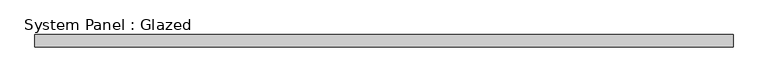
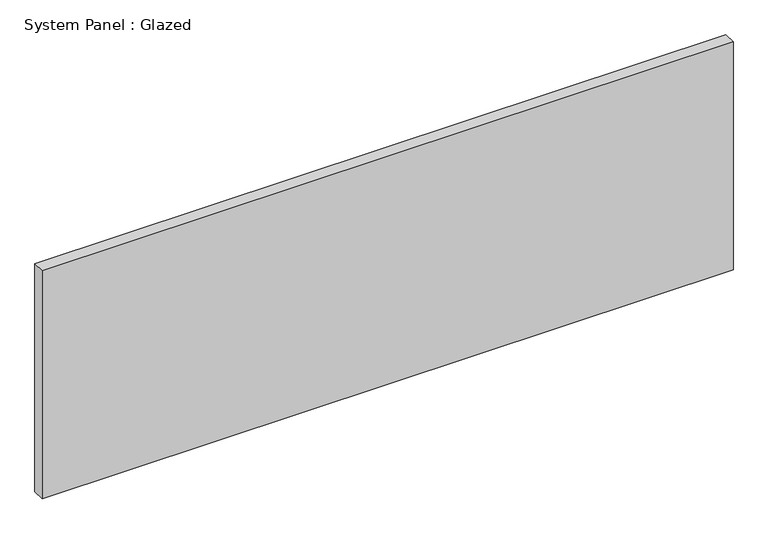
"""IFC4 building model written with IfcOpenShell, lengths in millimetres: plate geometry, System Panel : Glazed."""

from ifc_helpers import new_model, si_unit, origin, origin_with_axes, place, context, project, spatial, polyline, outline, extrude, source, transform, mapped, element, save


def system_panel_glazed_d4e05dc3(model_context):
    return source(origin(), model_context, "Body", "SweptSolid", [
        extrude(outline(polyline([(711.2, 19.05), (-711.2, 19.05), (-711.2, 44.45), (711.2, 44.45), (711.2, 19.05)])), origin_with_axes(), (0.0, 0.0, 1.0), 495.6398623),
    ])


if __name__ == "__main__":
    model = new_model("IFC4")
    model_context = context("Model", 3, world=origin())
    ifc_project = project(units=[si_unit("LENGTHUNIT", "METRE", prefix="MILLI")], contexts=[model_context])
    site = spatial("IfcSite", under=ifc_project)
    building = spatial("IfcBuilding", under=site)
    placement = place(None, origin())
    system_panel_glazed_shape = system_panel_glazed_d4e05dc3(model_context)
    element("IfcPlate", 1, ObjectType="System Panel : Glazed", at=placement, inside=building, context=model_context, shape_type="MappedRepresentation", body=[
        mapped(system_panel_glazed_shape, transform((0.0, 0.0, 0.0), x_axis=(1.0, 0.0, 0.0), y_axis=(0.0, 1.0, 0.0), z_axis=(0.0, 0.0, 1.0))),
    ])
    save(model, "model.ifc")

# Revit data of these elements
# Type "System Panel : Glazed"
#   Construction Type Id = "GSP4R"
#   Analytic Construction = "1/8 in Pilkington single glazing"
#   Visual Light Transmittance = 0.9
#   Solar Heat Gain Coefficient = 0.86
#   Heat Transfer Coefficient (U) = 1.18115 BTU/(h·ft²·°F)
#   Define Thermal Properties by = 1
# Element 1 (IfcPlate, "System Panel : Glazed")
#   Materials on its faces: "Glass"
# Materials
#   "Glass": class "Glass", colour RGB 0 128 192, transparency 0.75, Description = "Soda Lime Glass", Cost = 0
